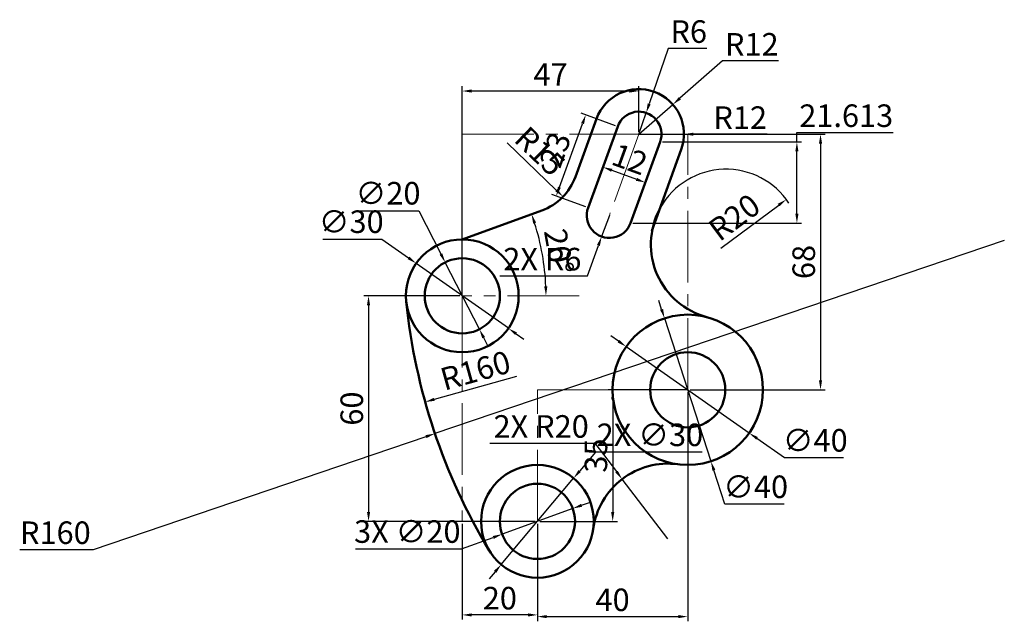
# Model space of a CAD drawing. Units: millimetres. Extents: x -10 to 252, y 18 to 178.
import ezdxf

# ---------------------------------------------------------------- set-up
doc = ezdxf.new("R2010")
doc.units = ezdxf.units.MM
doc.linetypes.add('CENTER2', pattern=[28.575, 19.05, -3.175, 3.175, -3.175])
for name, color, linetype, lineweight in [('M-CNTR', 4, 'CENTER2', 18), ('M-DIMS', 2, 'Continuous', 25), ('M-OUTL', 7, 'Continuous', 50)]:
    doc.layers.add(name, color=color, linetype=linetype, lineweight=lineweight)
doc.styles.get("Standard").update_dxf_attribs({"font": 'arial.ttf'})
doc.dimstyles.new('ISO-25', dxfattribs={"dimtxt": 6, "dimasz": 2.5, "dimexe": 1.25, "dimexo": 0.625, "dimtad": 1, "dimtoh": 1, "dimdec": 1, "dimtxsty": 'Standard', "dimcen": 2.5, "dimadec": 0, "dimazin": 0, "dimtfac": 1, "dimtdec": 1, "dimtmove": 0, "dimatfit": 3, "dimfxl": 1, "dimarcsym": 0})

# ---------------------------------------------------------------- blocks, each defined once
blk = doc.blocks.new('*D1')
at = {"layer": 'Defpoints', "color": 0, "transparency": 16777216}
for p in [(128.83, 127.31), (107.69, 119.62), (129.54, 111.99), (107.69, 104.62), (138.79, 104.62)]:
    blk.add_point(p, dxfattribs=at)
at = {"layer": 'M-DIMS', "color": 0, "lineweight": -2, "transparency": 16777216}
blk.add_arc((66.48, 104.62), 63.49, 2.2564, 17.7436, dxfattribs=at)
at = {"layer": 'M-DIMS', "color": 0, "transparency": 16777216}
for points in [[(126.55, 123.83), (127.34, 124.1), (126.14, 126.33)], [(130.33, 107.12), (129.5, 107.11), (129.96, 104.62)]]:
    blk.add_solid(points, dxfattribs=at)
at = {"layer": 'M-DIMS', "color": 0, "transparency": 16777216, "insert": (132.63, 116.28), "char_height": 6, "attachment_point": 5, "rotation": 280}
blk.add_mtext('20°', dxfattribs=at)
blk = doc.blocks.new('*D2')
at = {"layer": 'Defpoints', "color": 0, "transparency": 16777216}
for p in [(95.44, 113.26), (119.95, 95.97)]:
    blk.add_point(p, dxfattribs=at)
at = {"layer": 'M-DIMS', "color": 0, "lineweight": -2, "transparency": 16777216}
for p, q in [((70.58, 119.71), (86.31, 119.71)), ((86.31, 119.71), (93.39, 114.71)), ((119.95, 95.97), (95.44, 113.26)), ((121.99, 94.53), (124.03, 93.09))]:
    blk.add_line(p, q, dxfattribs=at)
at = {"layer": 'M-DIMS', "color": 0, "transparency": 16777216}
for points in [[(93.63, 115.05), (93.15, 114.37), (95.44, 113.26)], [(122.23, 94.87), (121.75, 94.19), (119.95, 95.97)]]:
    blk.add_solid(points, dxfattribs=at)
at = {"layer": 'M-DIMS', "color": 0, "transparency": 16777216, "insert": (78.13, 123.56), "char_height": 6, "attachment_point": 5}
blk.add_mtext('∅30', dxfattribs=at)
blk = doc.blocks.new('*D3')
at = {"layer": 'Defpoints', "color": 0, "transparency": 16777216}
for p in [(103.14, 113.52), (112.24, 95.71)]:
    blk.add_point(p, dxfattribs=at)
at = {"layer": 'M-DIMS', "color": 0, "lineweight": -2, "transparency": 16777216}
for p, q in [((80.38, 127.27), (96.11, 127.27)), ((96.11, 127.27), (102, 115.75)), ((112.24, 95.71), (103.14, 113.52)), ((113.38, 93.49), (114.52, 91.26))]:
    blk.add_line(p, q, dxfattribs=at)
at = {"layer": 'M-DIMS', "color": 0, "transparency": 16777216}
for points in [[(102.37, 115.94), (101.63, 115.56), (103.14, 113.52)], [(113.75, 93.68), (113.01, 93.3), (112.24, 95.71)]]:
    blk.add_solid(points, dxfattribs=at)
at = {"layer": 'M-DIMS', "color": 0, "transparency": 16777216, "insert": (87.93, 131.13), "char_height": 6, "attachment_point": 5}
blk.add_mtext('∅20', dxfattribs=at)
blk = doc.blocks.new('*D4')
at = {"layer": 'Defpoints', "color": 0, "transparency": 16777216}
for p in [(107.69, 159.1), (154.69, 147.62), (107.69, 104.62)]:
    blk.add_point(p, dxfattribs=at)
at = {"layer": 'M-DIMS', "color": 0, "lineweight": -2, "transparency": 16777216}
for p, q in [((107.69, 105.24), (107.69, 160.35)), ((154.69, 148.24), (154.69, 160.35)), ((152.19, 159.1), (110.19, 159.1))]:
    blk.add_line(p, q, dxfattribs=at)
at = {"layer": 'M-DIMS', "color": 0, "transparency": 16777216}
for points in [[(110.19, 159.52), (110.19, 158.68), (107.69, 159.1)], [(152.19, 159.52), (152.19, 158.68), (154.69, 159.1)]]:
    blk.add_solid(points, dxfattribs=at)
at = {"layer": 'M-DIMS', "color": 0, "transparency": 16777216, "insert": (131.19, 162.72), "char_height": 6, "attachment_point": 5}
blk.add_mtext('47', dxfattribs=at)
blk = doc.blocks.new('*D5')
at = {"layer": 'Defpoints', "color": 0, "transparency": 16777216}
for p in [(163.72, 155.52), (154.69, 147.62)]:
    blk.add_point(p, dxfattribs=at)
at = {"layer": 'M-DIMS', "color": 0, "lineweight": -2, "transparency": 16777216}
for p, q in [((176.96, 167.11), (165.6, 157.17)), ((191.86, 167.11), (176.96, 167.11)), ((154.69, 147.62), (163.72, 155.52))]:
    blk.add_line(p, q, dxfattribs=at)
at = {"layer": 'M-DIMS', "color": 0, "transparency": 16777216}
blk.add_solid([(165.33, 157.48), (165.88, 156.85), (163.72, 155.52)], dxfattribs=at)
at = {"layer": 'M-DIMS', "color": 0, "transparency": 16777216, "insert": (184.73, 170.75), "char_height": 6, "attachment_point": 5}
blk.add_mtext('R12', dxfattribs=at)
blk = doc.blocks.new('*D6')
at = {"layer": 'Defpoints', "color": 0, "transparency": 16777216}
for p in [(156.63, 153.3), (154.69, 147.62)]:
    blk.add_point(p, dxfattribs=at)
at = {"layer": 'M-DIMS', "color": 0, "lineweight": -2, "transparency": 16777216}
for p, q in [((162.49, 170.45), (157.44, 155.66)), ((172.78, 170.45), (162.49, 170.45)), ((154.69, 147.62), (156.63, 153.3))]:
    blk.add_line(p, q, dxfattribs=at)
at = {"layer": 'M-DIMS', "color": 0, "transparency": 16777216}
blk.add_solid([(157.04, 155.8), (157.83, 155.53), (156.63, 153.3)], dxfattribs=at)
at = {"layer": 'M-DIMS', "color": 0, "transparency": 16777216, "insert": (167.95, 174.14), "char_height": 6, "attachment_point": 5}
blk.add_mtext('R6', dxfattribs=at)
blk = doc.blocks.new('*D7')
at = {"layer": 'Defpoints', "color": 0, "transparency": 16777216}
for p in [(123.7, 141.41), (134.51, 131.01)]:
    blk.add_point(p, dxfattribs=at)
at = {"layer": 'M-DIMS', "color": 0, "lineweight": -2, "transparency": 16777216}
blk.add_line((119.64, 145.31), (132.71, 132.74), dxfattribs=at)
at = {"layer": 'M-DIMS', "color": 0, "transparency": 16777216}
blk.add_solid([(133, 133.04), (132.42, 132.44), (134.51, 131.01)], dxfattribs=at)
at = {"layer": 'M-DIMS', "color": 0, "transparency": 16777216, "insert": (127.83, 142.55), "char_height": 6, "attachment_point": 5, "rotation": 316.1099}
blk.add_mtext('R15', dxfattribs=at)
blk = doc.blocks.new('*D8')
at = {"layer": 'Defpoints', "color": 0, "transparency": 16777216}
for p in [(145.12, 138.86), (156.4, 134.76), (156.4, 134.76)]:
    blk.add_point(p, dxfattribs=at)
at = {"layer": 'M-DIMS', "color": 0, "lineweight": -2, "transparency": 16777216}
for p, q in [((145.33, 139.45), (145.55, 140.04)), ((147.47, 138.01), (154.05, 135.61)), ((156.61, 135.35), (156.82, 135.93))]:
    blk.add_line(p, q, dxfattribs=at)
at = {"layer": 'M-DIMS', "color": 0, "transparency": 16777216}
for points in [[(147.61, 138.4), (147.33, 137.62), (145.12, 138.86)], [(154.19, 136), (153.9, 135.22), (156.4, 134.76)]]:
    blk.add_solid(points, dxfattribs=at)
at = {"layer": 'M-DIMS', "color": 0, "transparency": 16777216, "insert": (152, 140.23), "char_height": 6, "attachment_point": 5, "rotation": 340}
blk.add_mtext('12', dxfattribs=at)
blk = doc.blocks.new('*D9')
at = {"layer": 'Defpoints', "color": 0, "transparency": 16777216}
for p in [(193.91, 130.26), (177.88, 118.3)]:
    blk.add_point(p, dxfattribs=at)
at = {"layer": 'M-DIMS', "color": 0, "lineweight": -2, "transparency": 16777216}
blk.add_line((176.52, 117.28), (191.91, 128.76), dxfattribs=at)
blk.add_arc((177.88, 118.3), 20, 33.1449, 150.5378, dxfattribs=at)
at = {"layer": 'M-DIMS', "color": 0, "transparency": 16777216}
blk.add_solid([(191.66, 129.1), (192.16, 128.43), (193.91, 130.26)], dxfattribs=at)
at = {"layer": 'M-DIMS', "color": 0, "transparency": 16777216, "insert": (180.55, 124.89), "char_height": 6, "attachment_point": 5, "rotation": 36.7259}
blk.add_mtext('R20', dxfattribs=at)
blk = doc.blocks.new('*D10')
at = {"layer": 'Defpoints', "color": 0, "transparency": 16777216}
for p in [(154.69, 147.62), (167.69, 79.62), (203.03, 79.62)]:
    blk.add_point(p, dxfattribs=at)
at = {"layer": 'M-DIMS', "color": 0, "lineweight": -2, "transparency": 16777216}
for p, q in [((155.32, 147.62), (204.28, 147.62)), ((203.03, 145.12), (203.03, 82.12)), ((168.32, 79.62), (204.28, 79.62))]:
    blk.add_line(p, q, dxfattribs=at)
at = {"layer": 'M-DIMS', "color": 0, "transparency": 16777216}
for points in [[(202.61, 145.12), (203.44, 145.12), (203.03, 147.62)], [(202.61, 82.12), (203.44, 82.12), (203.03, 79.62)]]:
    blk.add_solid(points, dxfattribs=at)
at = {"layer": 'M-DIMS', "color": 0, "transparency": 16777216, "insert": (199.34, 113.62), "char_height": 6, "attachment_point": 5, "rotation": 90}
blk.add_mtext('68', dxfattribs=at)
blk = doc.blocks.new('*D11')
at = {"layer": 'Defpoints', "color": 0, "transparency": 16777216}
for p in [(107.69, 44.62), (127.69, 44.62), (107.69, 19.73)]:
    blk.add_point(p, dxfattribs=at)
at = {"layer": 'M-DIMS', "color": 0, "lineweight": -2, "transparency": 16777216}
for p, q in [((107.69, 43.99), (107.69, 18.48)), ((127.69, 43.99), (127.69, 18.48)), ((125.19, 19.73), (110.19, 19.73))]:
    blk.add_line(p, q, dxfattribs=at)
at = {"layer": 'M-DIMS', "color": 0, "transparency": 16777216}
for points in [[(110.19, 20.14), (110.19, 19.31), (107.69, 19.73)], [(125.19, 20.14), (125.19, 19.31), (127.69, 19.73)]]:
    blk.add_solid(points, dxfattribs=at)
at = {"layer": 'M-DIMS', "color": 0, "transparency": 16777216, "insert": (117.69, 23.41), "char_height": 6, "attachment_point": 5}
blk.add_mtext('20', dxfattribs=at)
blk = doc.blocks.new('*D12')
at = {"layer": 'Defpoints', "color": 0, "transparency": 16777216}
for p in [(107.69, 104.62), (82.74, 44.62), (127.69, 44.62)]:
    blk.add_point(p, dxfattribs=at)
at = {"layer": 'M-DIMS', "color": 0, "lineweight": -2, "transparency": 16777216}
for p, q in [((107.07, 104.62), (81.49, 104.62)), ((82.74, 102.12), (82.74, 47.12)), ((127.07, 44.62), (81.49, 44.62))]:
    blk.add_line(p, q, dxfattribs=at)
at = {"layer": 'M-DIMS', "color": 0, "transparency": 16777216}
for points in [[(82.33, 102.12), (83.16, 102.12), (82.74, 104.62)], [(82.33, 47.12), (83.16, 47.12), (82.74, 44.62)]]:
    blk.add_solid(points, dxfattribs=at)
at = {"layer": 'M-DIMS', "color": 0, "transparency": 16777216, "insert": (79.06, 74.62), "char_height": 6, "attachment_point": 5, "rotation": 90}
blk.add_mtext('60', dxfattribs=at)
blk = doc.blocks.new('*D13')
at = {"layer": 'Defpoints', "color": 0, "transparency": 16777216}
for p in [(167.69, 79.62), (127.69, 44.62), (167.69, 19.28)]:
    blk.add_point(p, dxfattribs=at)
at = {"layer": 'M-DIMS', "color": 0, "lineweight": -2, "transparency": 16777216}
for p, q in [((167.69, 78.99), (167.69, 18.03)), ((127.69, 43.99), (127.69, 18.03)), ((130.19, 19.28), (165.19, 19.28))]:
    blk.add_line(p, q, dxfattribs=at)
at = {"layer": 'M-DIMS', "color": 0, "transparency": 16777216}
for points in [[(130.19, 19.7), (130.19, 18.86), (127.69, 19.28)], [(165.19, 19.7), (165.19, 18.86), (167.69, 19.28)]]:
    blk.add_solid(points, dxfattribs=at)
at = {"layer": 'M-DIMS', "color": 0, "transparency": 16777216, "insert": (147.69, 22.97), "char_height": 6, "attachment_point": 5}
blk.add_mtext('40', dxfattribs=at)
blk = doc.blocks.new('*D14')
at = {"layer": 'Defpoints', "color": 0, "transparency": 16777216}
for p in [(151.32, 91.1), (184.06, 68.13)]:
    blk.add_point(p, dxfattribs=at)
at = {"layer": 'M-DIMS', "color": 0, "lineweight": -2, "transparency": 16777216}
for p, q in [((149.27, 92.54), (147.23, 93.98)), ((151.32, 91.1), (184.06, 68.13)), ((193.45, 61.55), (186.11, 66.69)), ((209.17, 61.55), (193.45, 61.55))]:
    blk.add_line(p, q, dxfattribs=at)
at = {"layer": 'M-DIMS', "color": 0, "transparency": 16777216}
for points in [[(149.51, 92.88), (149.03, 92.2), (151.32, 91.1)], [(186.35, 67.03), (185.87, 66.35), (184.06, 68.13)]]:
    blk.add_solid(points, dxfattribs=at)
at = {"layer": 'M-DIMS', "color": 0, "transparency": 16777216, "insert": (201.62, 65.4), "char_height": 6, "attachment_point": 5}
blk.add_mtext('∅40', dxfattribs=at)
blk = doc.blocks.new('*D15')
at = {"layer": 'Defpoints', "color": 0, "transparency": 16777216}
for p in [(167.69, 79.62), (127.69, 44.62), (147.72, 44.62)]:
    blk.add_point(p, dxfattribs=at)
at = {"layer": 'M-DIMS', "color": 0, "lineweight": -2, "transparency": 16777216}
for p, q in [((167.07, 79.62), (146.47, 79.62)), ((147.72, 77.12), (147.72, 47.12)), ((128.32, 44.62), (148.97, 44.62))]:
    blk.add_line(p, q, dxfattribs=at)
at = {"layer": 'M-DIMS', "color": 0, "transparency": 16777216}
for points in [[(147.3, 77.12), (148.14, 77.12), (147.72, 79.62)], [(147.3, 47.12), (148.14, 47.12), (147.72, 44.62)]]:
    blk.add_solid(points, dxfattribs=at)
at = {"layer": 'M-DIMS', "color": 0, "transparency": 16777216, "insert": (144.03, 62.12), "char_height": 6, "attachment_point": 5, "rotation": 90}
blk.add_mtext('35', dxfattribs=at)
blk = doc.blocks.new('*D16')
at = {"layer": 'Defpoints', "color": 0, "transparency": 16777216}
for p in [(251.94, 119.37), (97.82, 76.4)]:
    blk.add_point(p, dxfattribs=at)
at = {"layer": 'M-DIMS', "color": 0, "lineweight": -2, "transparency": 16777216}
blk.add_line((122.12, 83.17), (100.23, 77.07), dxfattribs=at)
at = {"layer": 'M-DIMS', "color": 0, "transparency": 16777216}
blk.add_solid([(100.11, 77.47), (100.34, 76.67), (97.82, 76.4)], dxfattribs=at)
at = {"layer": 'M-DIMS', "color": 0, "transparency": 16777216, "insert": (111.39, 84.01), "char_height": 6, "attachment_point": 5, "rotation": 15.5782}
blk.add_mtext('R160', dxfattribs=at)
blk = doc.blocks.new('HOLE-D20-OD30')
for radius in [15, 10]:
    blk.add_circle((15, 15), radius)
blk = doc.blocks.new('*D18')
at = {"layer": 'Defpoints', "color": 0, "transparency": 16777216}
for p in [(140.55, 152.76), (149.05, 149.67), (141.19, 128.06)]:
    blk.add_point(p, dxfattribs=at)
at = {"layer": 'M-DIMS', "color": 0, "lineweight": -2, "transparency": 16777216}
for p, q in [((148.47, 149.88), (139.37, 153.19)), ((133.54, 133.5), (139.69, 150.41)), ((140.6, 128.27), (131.51, 131.58))]:
    blk.add_line(p, q, dxfattribs=at)
at = {"layer": 'M-DIMS', "color": 0, "transparency": 16777216}
for points in [[(139.3, 150.56), (140.09, 150.27), (140.55, 152.76)], [(133.15, 133.64), (133.93, 133.36), (132.68, 131.15)]]:
    blk.add_solid(points, dxfattribs=at)
at = {"layer": 'M-DIMS', "color": 0, "transparency": 16777216, "insert": (133.15, 143.22), "char_height": 6, "attachment_point": 5, "rotation": 70}
blk.add_mtext('23', dxfattribs=at)
blk = doc.blocks.new('*D19')
at = {"layer": 'Defpoints', "color": 0, "transparency": 16777216}
for p in [(160.33, 145.56), (196.74, 145.56), (152.46, 123.95)]:
    blk.add_point(p, dxfattribs=at)
at = {"layer": 'M-DIMS', "color": 0, "lineweight": -2, "transparency": 16777216}
for p, q in [((196.74, 145.56), (196.74, 148.06)), ((196.74, 148.06), (222.38, 148.06)), ((160.95, 145.56), (197.99, 145.56)), ((196.74, 126.45), (196.74, 143.06)), ((153.09, 123.95), (197.99, 123.95))]:
    blk.add_line(p, q, dxfattribs=at)
at = {"layer": 'M-DIMS', "color": 0, "transparency": 16777216}
for points in [[(196.33, 143.06), (197.16, 143.06), (196.74, 145.56)], [(196.33, 126.45), (197.16, 126.45), (196.74, 123.95)]]:
    blk.add_solid(points, dxfattribs=at)
at = {"layer": 'M-DIMS', "color": 0, "transparency": 16777216, "insert": (209.87, 151.76), "char_height": 6, "attachment_point": 5}
blk.add_mtext('21.613', dxfattribs=at)
blk = doc.blocks.new('*D20')
at = {"layer": 'Defpoints', "color": 0, "transparency": 16777216}
for p in [(161.51, 98.64), (173.87, 60.6)]:
    blk.add_point(p, dxfattribs=at)
at = {"layer": 'M-DIMS', "color": 0, "lineweight": -2, "transparency": 16777216}
for p, q in [((160.74, 101.02), (159.97, 103.39)), ((161.51, 98.64), (173.87, 60.6)), ((177.58, 49.18), (174.65, 58.22)), ((193.31, 49.18), (177.58, 49.18))]:
    blk.add_line(p, q, dxfattribs=at)
at = {"layer": 'M-DIMS', "color": 0, "transparency": 16777216}
for points in [[(161.13, 101.14), (160.34, 100.89), (161.51, 98.64)], [(175.04, 58.35), (174.25, 58.09), (173.87, 60.6)]]:
    blk.add_solid(points, dxfattribs=at)
at = {"layer": 'M-DIMS', "color": 0, "transparency": 16777216, "insert": (185.76, 53.04), "char_height": 6, "attachment_point": 5}
blk.add_mtext('∅40', dxfattribs=at)
blk = doc.blocks.new('*D21')
at = {"layer": 'Defpoints', "color": 0, "transparency": 16777216}
for p in [(137.09, 48.04), (118.29, 41.2)]:
    blk.add_point(p, dxfattribs=at)
at = {"layer": 'M-DIMS', "color": 0, "lineweight": -2, "transparency": 16777216}
for p, q in [((137.09, 48.04), (118.29, 41.2)), ((139.44, 48.89), (141.79, 49.75)), ((107.52, 37.28), (115.95, 40.34)), ((79.23, 37.28), (107.52, 37.28))]:
    blk.add_line(p, q, dxfattribs=at)
at = {"layer": 'M-DIMS', "color": 0, "transparency": 16777216}
for points in [[(139.3, 49.28), (139.58, 48.5), (137.09, 48.04)], [(115.8, 40.73), (116.09, 39.95), (118.29, 41.2)]]:
    blk.add_solid(points, dxfattribs=at)
at = {"layer": 'M-DIMS', "color": 0, "transparency": 16777216, "insert": (93.06, 41.13), "char_height": 6, "attachment_point": 5}
blk.add_mtext('3X ∅20', dxfattribs=at)
blk = doc.blocks.new('*D22')
at = {"layer": 'Defpoints', "color": 0, "transparency": 16777216}
for p in [(137.33, 56.11), (118.05, 33.13)]:
    blk.add_point(p, dxfattribs=at)
at = {"layer": 'M-DIMS', "color": 0, "lineweight": -2, "transparency": 16777216}
for p, q in [((143.12, 63), (138.94, 58.02)), ((171.52, 63), (143.12, 63)), ((118.05, 33.13), (137.33, 56.11)), ((116.44, 31.21), (114.84, 29.3))]:
    blk.add_line(p, q, dxfattribs=at)
at = {"layer": 'M-DIMS', "color": 0, "transparency": 16777216}
for points in [[(138.62, 58.29), (139.26, 57.75), (137.33, 56.11)], [(116.12, 31.48), (116.76, 30.94), (118.05, 33.13)]]:
    blk.add_solid(points, dxfattribs=at)
at = {"layer": 'M-DIMS', "color": 0, "transparency": 16777216, "insert": (157.63, 66.86), "char_height": 6, "attachment_point": 5}
blk.add_mtext('2X ∅30', dxfattribs=at)
blk = doc.blocks.new('*D23')
at = {"layer": 'Defpoints', "color": 0, "transparency": 16777216}
for p in [(150.24, 55.86), (162.38, 39.97)]:
    blk.add_point(p, dxfattribs=at)
at = {"layer": 'M-DIMS', "color": 0, "lineweight": -2, "transparency": 16777216}
for p, q in [((115.02, 65.4), (142.96, 65.4)), ((142.96, 65.4), (148.72, 57.85)), ((162.38, 39.97), (150.24, 55.86))]:
    blk.add_line(p, q, dxfattribs=at)
at = {"layer": 'M-DIMS', "color": 0, "transparency": 16777216}
blk.add_solid([(149.06, 58.1), (148.39, 57.6), (150.24, 55.86)], dxfattribs=at)
at = {"layer": 'M-DIMS', "color": 0, "transparency": 16777216, "insert": (128.68, 69.09), "char_height": 6, "attachment_point": 5}
blk.add_mtext('2X R20', dxfattribs=at)
blk = doc.blocks.new('*D24')
at = {"layer": 'Defpoints', "color": 0, "transparency": 16777216}
for p in [(154.69, 147.62), (166.69, 147.62)]:
    blk.add_point(p, dxfattribs=at)
at = {"layer": 'M-DIMS', "color": 0, "lineweight": -2, "transparency": 16777216}
for p, q in [((154.69, 147.62), (166.69, 147.62)), ((173.89, 147.62), (169.19, 147.62)), ((188.79, 147.62), (173.89, 147.62))]:
    blk.add_line(p, q, dxfattribs=at)
at = {"layer": 'M-DIMS', "color": 0, "transparency": 16777216}
blk.add_solid([(169.19, 148.03), (169.19, 147.2), (166.69, 147.62)], dxfattribs=at)
at = {"layer": 'M-DIMS', "color": 0, "transparency": 16777216, "insert": (181.65, 151.25), "char_height": 6, "attachment_point": 5}
blk.add_mtext('R12', dxfattribs=at)
blk = doc.blocks.new('*D25')
at = {"layer": 'Defpoints', "color": 0, "transparency": 16777216}
for p in [(146.83, 126), (144.77, 120.37)]:
    blk.add_point(p, dxfattribs=at)
at = {"layer": 'M-DIMS', "color": 0, "lineweight": -2, "transparency": 16777216}
for p, q in [((146.83, 126), (144.77, 120.37)), ((140.97, 109.91), (143.92, 118.02)), ((117.68, 109.91), (140.97, 109.91))]:
    blk.add_line(p, q, dxfattribs=at)
at = {"layer": 'M-DIMS', "color": 0, "transparency": 16777216}
blk.add_solid([(143.53, 118.16), (144.31, 117.87), (144.77, 120.37)], dxfattribs=at)
at = {"layer": 'M-DIMS', "color": 0, "transparency": 16777216, "insert": (129.01, 113.6), "char_height": 6, "attachment_point": 5}
blk.add_mtext('2X R6', dxfattribs=at)
blk = doc.blocks.new('*D26')
at = {"layer": 'Defpoints', "color": 0, "transparency": 16777216}
for p in [(251.94, 119.37), (100.42, 67.97)]:
    blk.add_point(p, dxfattribs=at)
at = {"layer": 'M-DIMS', "color": 0, "lineweight": -2, "transparency": 16777216}
for p, q in [((251.94, 119.37), (100.42, 67.97)), ((9.51, 37.14), (98.05, 67.17)), ((-10.1, 37.14), (9.51, 37.14))]:
    blk.add_line(p, q, dxfattribs=at)
at = {"layer": 'M-DIMS', "color": 0, "transparency": 16777216}
blk.add_solid([(97.92, 67.56), (98.18, 66.77), (100.42, 67.97)], dxfattribs=at)
at = {"layer": 'M-DIMS', "color": 0, "transparency": 16777216, "insert": (-0.61, 40.82), "char_height": 6, "attachment_point": 5}
blk.add_mtext('R160', dxfattribs=at)

msp = doc.modelspace()

# ---------------------------------------------------------------- linework, layer by layer
at = {"layer": 'M-CNTR'}
for points in [[(138.7911, 104.6168), (107.6917, 104.6168), (107.6917, 147.6168), (154.6917, 147.6168), (146.8253, 126.0038)], [(107.6917, 104.6168), (107.6917, 44.6168), (127.6917, 44.6168), (127.6917, 79.6168), (167.6917, 79.6168), (167.6917, 147.6168)]]:
    msp.add_lwpolyline(points, dxfattribs=at)
at = {"layer": 'M-OUTL'}
msp.add_lwpolyline([(107.6917, 119.6168), (128.8284, 127.3099, 0.22169466), (137.7935, 136.275), (143.4154, 151.721, -1), (165.968, 143.5125), (158.1016, 121.8996)], format="xyb", dxfattribs=at)
msp.add_lwpolyline([(149.0536, 149.6689), (141.1871, 128.056, 1), (152.4634, 123.9517), (160.3299, 145.5646, 1)], format="xyb", close=True, dxfattribs=at)
for radius in [20, 10]:
    msp.add_circle((167.6917, 79.6168), radius, dxfattribs=at)
for centre, radius, start, end in [((177.8833, 118.2966), 20, 152.32832, 255.238957), ((251.9396, 119.3661), 160, 185.838185, 211.031712), ((162.382, 39.9707), 20, 82.37185, 172.37185)]:
    msp.add_arc(centre, radius, start, end, dxfattribs=at)

# ---------------------------------------------------------------- block references
for p in [(92.692, 89.617), (112.692, 29.617)]:
    msp.add_blockref('HOLE-D20-OD30', p, dxfattribs=at)

# ---------------------------------------------------------------- dimensions: what is measured, and where the dimension line sits
at = {"layer": 'M-DIMS'}
for center, mpoint, override, picture, middle in [((154.6917, 147.6168), (156.6299, 153.2951), {"dimclrd": 0, "dimclre": 0, "dimclrt": 0}, '*D6', (167.9463, 170.4507)), ((154.6917, 147.6168), (163.7212, 155.5205), {"dimclrd": 0, "dimclre": 0, "dimclrt": 0}, '*D5', (184.7269, 167.1122)), ((154.6917, 147.6168), (166.6917, 147.617), {"dimdec": 0, "dimlfac": 1, "dimrnd": 0, "dimzin": 0, "dimdsep": 46, "dimlunit": 2}, '*D24', (173.8917, 147.6171)), ((123.6981, 141.4053), (134.5082, 131.0061), {"dimclrd": 0, "dimclre": 0, "dimclrt": 0}, '*D7', (125.2721, 139.8912)), ((177.8833, 118.2966), (193.9134, 130.2564), {"dimclrd": 0, "dimclre": 0, "dimclrt": 0}, '*D9', (182.7555, 121.9317)), ((251.9396, 119.3661), (100.4184, 67.9723), {"dimdec": 0, "dimlfac": 1, "dimrnd": 0, "dimzin": 0, "dimdsep": 46, "dimlunit": 2}, '*D26', (-0.6084, 37.1361)), ((251.9396, 119.3661), (97.8173, 76.3974), {"dimclrd": 0, "dimclre": 0, "dimclrt": 0}, '*D16', (112.3761, 80.4564))]:
    dim = msp.add_radius_dim(center=center, mpoint=mpoint, dimstyle='ISO-25', override=override, dxfattribs=at)
    dim.commit()
    dim.dimension.update_dxf_attribs({"geometry": picture, "text_midpoint": middle, "dimtype": 164})
for base, p1, p2, picture, middle in [((107.6917, 159.0999), (154.6917, 147.6168), (107.6917, 104.6168), '*D4', (131.1917, 162.7249)), ((167.6917, 19.2811), (127.6917, 44.6168), (167.6917, 79.6168), '*D13', (147.6917, 22.9696)), ((107.6917, 19.7262), (127.6917, 44.6168), (107.6917, 44.6168), '*D11', (117.6917, 23.4147))]:
    dim = msp.add_linear_dim(base=base, p1=p1, p2=p2, dimstyle='ISO-25', override={"dimclrd": 0, "dimclre": 0, "dimclrt": 0}, dxfattribs=at)
    dim.commit()
    dim.dimension.update_dxf_attribs({"geometry": picture, "text_midpoint": middle})
for base, p1, p2, angle, override, picture, middle in [((196.7417, 145.5646), (152.4634, 123.9517), (160.3299, 145.5646), 90, {"dimdec": 3, "dimlfac": 1, "dimrnd": 0, "dimzin": 0, "dimdsep": 46, "dimlunit": 2}, '*D19', (209.8722, 151.7551)), ((140.5493, 152.7642), (141.1871, 128.056), (149.0536, 149.6689), 70, {"dimdec": 0, "dimlfac": 1, "dimrnd": 0, "dimzin": 0, "dimdsep": 46, "dimlunit": 2}, '*D18', (133.1482, 143.2199)), ((203.0253, 79.6168), (154.6917, 147.6168), (167.6917, 79.6168), 90, {"dimclrd": 0, "dimclre": 0, "dimclrt": 0}, '*D10', (199.3368, 113.6168)), ((82.7444, 44.6168), (107.6917, 104.6168), (127.6917, 44.6168), 90, {"dimclrd": 0, "dimclre": 0, "dimclrt": 0}, '*D12', (79.056, 74.6168)), ((147.7185, 44.6168), (167.6917, 79.6168), (127.6917, 44.6168), 90, {"dimclrd": 0, "dimclre": 0, "dimclrt": 0}, '*D15', (144.028, 62.1168))]:
    dim = msp.add_linear_dim(base=base, p1=p1, p2=p2, angle=angle, dimstyle='ISO-25', override=override, dxfattribs=at)
    dim.commit()
    dim.dimension.update_dxf_attribs({"geometry": picture, "text_midpoint": middle})
dim = msp.add_aligned_dim(p1=(145.1203, 138.8624), p2=(156.3966, 134.7582), distance=0, dimstyle='ISO-25', override={"dimclrd": 0, "dimclre": 0, "dimclrt": 0}, dxfattribs=at)
dim.commit()
dim.dimension.update_dxf_attribs({"geometry": '*D8', "text_midpoint": (152.0025, 140.2282)})
for p1, p2, override, picture, middle in [((112.2441, 95.7131), (103.1393, 113.5205), {"dimclrd": 0, "dimclre": 0, "dimclrt": 0}, '*D3', (87.9315, 127.2732)), ((119.9478, 95.9688), (95.4356, 113.2648), {"dimclrd": 0, "dimclre": 0, "dimclrt": 0}, '*D2', (78.1308, 119.7061)), ((161.5104, 98.6376), (173.873, 60.5959), {"dimdec": 0, "dimlfac": 1, "dimrnd": 0, "dimzin": 0, "dimdsep": 46, "dimlunit": 2}, '*D20', (185.758, 49.1835))]:
    dim = msp.add_diameter_dim_2p(p1=p1, p2=p2, dimstyle='ISO-25', override=override, dxfattribs=at)
    dim.commit()
    dim.dimension.update_dxf_attribs({"geometry": picture, "text_midpoint": middle, "dimtype": 163})
dim = msp.add_angular_dim_2l(base=(129.5357, 111.987), line1=((138.7911, 104.6168), (107.6917, 104.6168)), line2=((107.6917, 119.6168), (128.8284, 127.3099)), dimstyle='ISO-25', override={"dimclrd": 0, "dimclre": 0, "dimclrt": 0}, dxfattribs=at)
dim.commit()
dim.dimension.update_dxf_attribs({"geometry": '*D1', "text_midpoint": (132.6328, 116.2814)})
dim = msp.add_radius_dim(center=(146.8253, 126.0038), mpoint=(144.7729, 120.3658), text='2X <>', dimstyle='ISO-25', override={"dimdec": 0, "dimlfac": 1, "dimrnd": 0, "dimzin": 0, "dimdsep": 46, "dimlunit": 2}, dxfattribs=at)
dim.commit()
dim.dimension.update_dxf_attribs({"geometry": '*D25', "text_midpoint": (129.009, 113.5985)})
dim = msp.add_diameter_dim_2p(p1=(151.3197, 91.1041), p2=(184.0637, 68.1295), dimstyle='ISO-25', override={"dimclrd": 0, "dimclre": 0, "dimclrt": 0}, dxfattribs=at)
dim.commit()
dim.dimension.update_dxf_attribs({"geometry": '*D14', "text_midpoint": (201.623, 65.402)})
dim = msp.add_radius_dim(center=(162.382, 39.9707), mpoint=(150.2421, 55.8649), text='2X <>', dimstyle='ISO-25', override={"dimdec": 0, "dimlfac": 1, "dimrnd": 0, "dimzin": 0, "dimdsep": 46, "dimlunit": 2}, dxfattribs=at)
dim.commit()
dim.dimension.update_dxf_attribs({"geometry": '*D23', "text_midpoint": (128.6776, 65.4013), "dimtype": 164})
for p1, p2, text, picture, middle in [((118.0499, 33.1261), (137.3335, 56.1074), '2X <>', '*D22', (157.6324, 63.0018)), ((137.0888, 48.0366), (118.2947, 41.1969), '3X <>', '*D21', (93.0627, 37.2768))]:
    dim = msp.add_diameter_dim_2p(p1=p1, p2=p2, text=text, dimstyle='ISO-25', override={"dimdec": 0, "dimlfac": 1, "dimrnd": 0, "dimzin": 0, "dimdsep": 46, "dimlunit": 2}, dxfattribs=at)
    dim.commit()
    dim.dimension.update_dxf_attribs({"geometry": picture, "text_midpoint": middle, "dimtype": 163})

doc.saveas('drawing.dxf')
